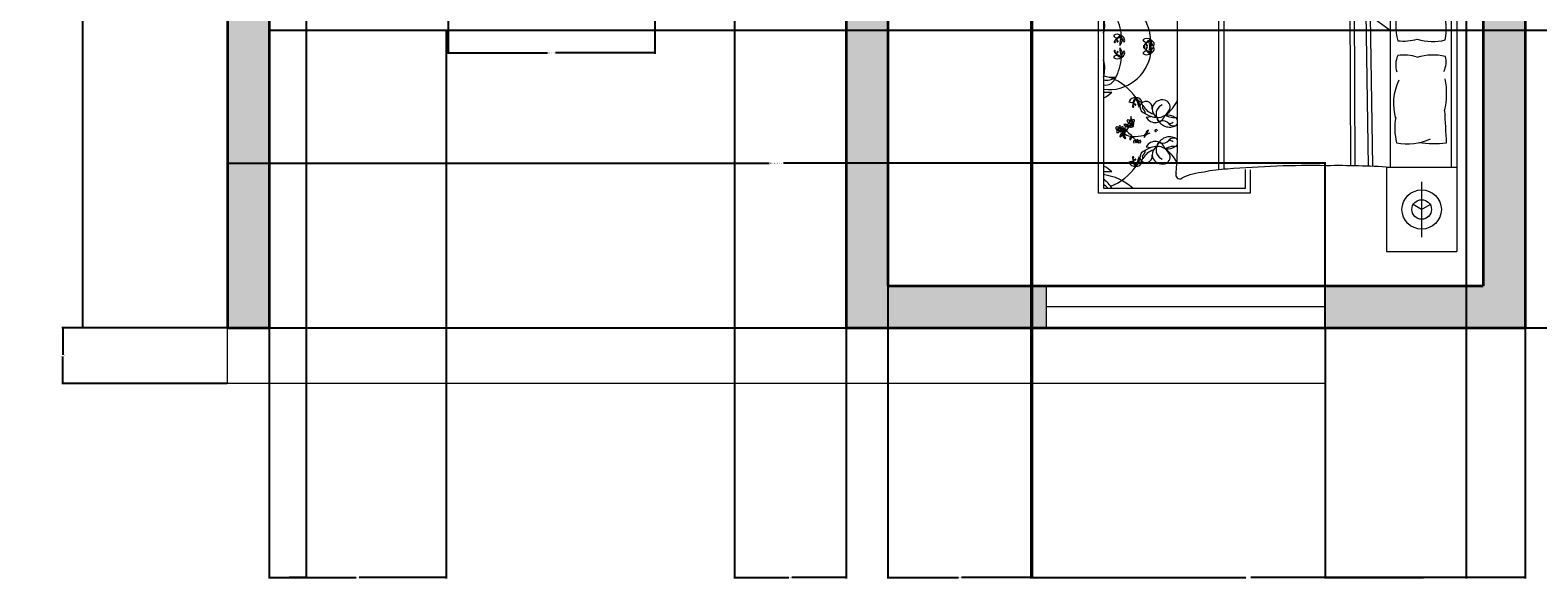
# Model space of a CAD drawing. Units: inches. Extents: x 37 to 706, y -568 to 110.
# Tile 1 of 24: x 37 to 361, y -568 to -450. Entities that reach past the tile are written whole.
import ezdxf

# ---------------------------------------------------------------- set-up
doc = ezdxf.new("R2010")
doc.units = ezdxf.units.IN
doc.header["$MEASUREMENT"] = 0
for name, color, linetype, lineweight in [('A-ANNO-DIMS', 2, 'Continuous', 18), ('A-FLOR-STRS', 7, 'Continuous', 18), ('A-FURN', 8, 'Continuous', 13), ('A-GLAZ', 4, 'Continuous', 18), ('A-WALL', 7, 'Continuous', 35), ('A-WALL-PATT', 252, 'Continuous', 13)]:
    doc.layers.add(name, color=color, linetype=linetype, lineweight=lineweight)
doc.styles.get("Standard").update_dxf_attribs({"font": 'arial.ttf'})
doc.dimstyles.get("Standard").update_dxf_attribs({"dimtxt": 0.18, "dimasz": 0.18, "dimexe": 0.18, "dimexo": 0.0625, "dimgap": 0.09, "dimtad": 0, "dimtih": 1, "dimtoh": 1, "dimdec": 0, "dimzin": 0, "dimdsep": 46, "dimlunit": 3, "dimtxsty": 'Standard', "dimcen": 0.09, "dimadec": 0, "dimazin": 0, "dimtfac": 1, "dimtdec": 0, "dimtofl": 0, "dimtmove": 0, "dimatfit": 3, "dimfxl": 1, "dimtolj": 1, "dimtzin": 0, "dimarcsym": 0})

# ---------------------------------------------------------------- blocks, each defined once
blk = doc.blocks.new('*D3')
at = {"layer": 'A-ANNO-DIMS', "color": 0, "lineweight": -2, "transparency": 16777216}
for p, q in [((78.9, 51.29), (47.67, 51.29)), ((47.85, 51.11), (47.85, -228.11)), ((47.85, -513.53), (47.85, -234.31)), ((78.9, -513.71), (47.67, -513.71))]:
    blk.add_line(p, q, dxfattribs=at)
at = {"layer": 'A-ANNO-DIMS', "color": 0, "transparency": 16777216}
for points in [[(47.82, 51.11), (47.88, 51.11), (47.85, 51.29)], [(47.82, -513.53), (47.88, -513.53), (47.85, -513.71)]]:
    blk.add_solid(points, dxfattribs=at)
at = {"layer": 'Defpoints', "color": 0, "transparency": 16777216}
for p in [(78.96, 51.29), (47.85, -513.71), (78.96, -513.71)]:
    blk.add_point(p, dxfattribs=at)
at = {"layer": 'A-ANNO-DIMS', "color": 0, "transparency": 16777216, "insert": (47.85, -231.21), "char_height": 6, "attachment_point": 5}
blk.add_mtext('\\A1;47\'-1"', dxfattribs=at)
blk = doc.blocks.new('BED-DOUBLE-WITH-NIGHTSTANDS')
for p, q in [((77.02, 90.57), (77.02, 0)), ((69.47, 75.59), (69.47, 87.43)), ((63.56, 81.51), (75.39, 81.51)), ((0, 78.61), (32.62, 78.61)), ((0, 12.59), (0, 78.61)), ((32.62, 78.61), (32.62, 73.49)), ((1.05, 77.56), (1.05, 13.64)), ((31.58, 77.56), (1.05, 77.56)), ((31.58, 73.49), (31.58, 77.56)), ((25.85, 17.62), (25.85, 73.5)), ((26.98, 17.7), (26.98, 73.5)), ((50.48, 72.53), (51.22, 73.26)), ((50.85, 68.86), (50.48, 72.53)), ((51.22, 73.26), (55.07, 69.96)), ((77.02, 72.45), (52.16, 72.45)), ((62.71, 72.45), (62.71, 18.11)), ((75.86, 18.11), (75.86, 72.45)), ((10.23, 68.64), (11.25, 68.84)), ((50.48, 64.28), (50.85, 68.86)), ((55.07, 69.96), (57.63, 66.48)), ((57.63, 66.48), (60.02, 59.87)), ((10.23, 62.31), (11.25, 62.11)), ((16.95, 26.9), (16.95, 63.67)), ((49.93, 60.24), (50.48, 64.28)), ((48.83, 57.86), (49.93, 60.24)), ((60.02, 59.87), (62.71, 50)), ((48.1, 54.92), (48.83, 57.86)), ((50.48, 54.55), (48.1, 54.92)), ((55.8, 52.54), (50.48, 54.55)), ((54.24, 18.43), (54.09, 53.18)), ((55.17, 18.44), (55.03, 52.83)), ((62.71, 47.57), (55.8, 52.54)), ((58.02, 18.39), (57.55, 51.28)), ((58.95, 18.36), (58.49, 50.6)), ((10.23, 28.89), (11.25, 29.09)), ((10.23, 22.56), (11.25, 22.36)), ((31.58, 13.64), (31.58, 17.63)), ((32.62, 17.61), (32.62, 12.59)), ((1.05, 13.64), (31.58, 13.64)), ((69.47, 14.97), (69.47, 3.14)), ((32.62, 12.59), (0, 12.59))]:
    blk.add_line(p, q)
for points in [[(61.93, 72.45), (61.93, 90.57), (77.02, 90.57)], [(69.47, 81.51), (67.64, 80.45)], [(69.47, 81.51), (71.3, 80.45)], [(77.02, 18.11), (61.93, 18.11), (61.93, 0), (77.02, 0)], [(69.47, 9.06), (67.64, 10.11)], [(69.47, 9.06), (71.3, 10.11)]]:
    blk.add_lwpolyline(points)
for points in [[(42.92, 73.45, 0.001242), (25.74, 73.5, -0.127202), (17.18, 75.31)], [(74.76, 67.25, 0.074897), (68.85, 67.14, -0.472817)], [(68.52, 45.71, 0.14099), (74.55, 45.53, 0.235245)], [(68.52, 41.84, -0.14099), (74.55, 42.02, -0.235245)], [(74.76, 23.32, -0.074897), (68.85, 23.42, 0.472817)], [(27.69, 17.73, 0.056112), (22.71, 17.07, 0.095341), (17.91, 15.8)]]:
    blk.add_lwpolyline(points, format="xyb")
for centre, radius in [((69.47, 81.51), 4.23), ((69.47, 81.51), 2.11), ((4.52, 64.91), 0.231), ((6.95, 63.41), 0.231), ((4.52, 26.28), 0.231), ((6.95, 27.79), 0.231), ((69.47, 9.06), 4.23), ((69.47, 9.06), 2.11)]:
    blk.add_circle(centre, radius)
for centre, radius, start, end in [((-3.2, 82.51), 7.18, 306.3036, 316.4814), ((-2.13, 80.43), 5.76, 303.4617, 330.1116), ((-0.54, 86.37), 11.83, 277.745, 311.8856), ((-1.71, 66.13), 11.83, 34.3865, 68.5908), ((17.23, 74.48), 0.836, 93.98, 207.3412), ((-0.79, 77.21), 4.81, 292.5547, 318.9546), ((1.79, 90.38), 16.36, 267.4081, 273.6519), ((7.77, 71.53), 1.31, 77.7115, 159.0387), ((7.06, 72.84), 0.988, 238.4633, 358.2869), ((10.3, 70.85), 2.99, 138.8402, 177.9352), ((8.5, 71.96), 0.967, 117.6827, 223.7762), ((7.89, 71.38), 0.128, 223.7762, 159.7183), ((8.28, 71.86), 0.98, 2.9516, 103.728), ((16.12, 74.61), 8.27, 192.5173, 207.1824), ((6.95, 71.3), 1.87, 345.4653, 54.2343), ((9.77, 73.87), 2.02, 211.3827, 255.2969), ((10.16, 70.71), 1.36, 350.264, 160.8688), ((8.69, 70.99), 0.833, 333.9755, 53.2681), ((13.65, 70.21), 2.16, 84.9449, 172.8857), ((14.47, 69.36), 2.1, 111.5819, 201.4221), ((13.86, 70.84), 1.53, 354.4856, 91.0538), ((10.57, 74.83), 6.85, 303.6671, 333.2997), ((-77.32, 64.75), 94.28, 359.3433, 5.6887), ((48.97, 156.3), 83.07, 265.8294, 271.553), ((83.29, 71.71), 34.18, 177.4519, 191.3392), ((7.46, 70.95), 0.147, 177.9352, 11.4834), ((7.53, 70.96), 0.0713, 11.4834, 127.9409), ((10.57, 71.04), 1.7, 175.969, 254.3045), ((8.31, 69.21), 1.81, 6.1662, 51.5825), ((13.15, 73.4), 4.28, 211.2614, 251.7045), ((12.81, 73.44), 4.86, 236.2883, 266.5076), ((12.18, 69.76), 2.25, 209.9085, 343.1337), ((14.13, 70.59), 2.63, 182.3591, 234.0401), ((12.73, 71.31), 2.72, 265.2933, 346.921), ((13.13, 68.34), 0.562, 167.3041, 285.1471), ((14.65, 65.65), 3.49, 122.7011, 126.3445), ((15.31, 69.41), 2.89, 199.2822, 299.1751), ((16.28, 72.32), 3.75, 238.8218, 279.1554), ((14.65, 65.65), 3.49, 55.785, 94.7304), ((15.95, 67.67), 1.09, 30.0293, 52.325), ((4.09, 64.6), 0.381, 61.2196, 169.0403), ((4.34, 65.38), 0.455, 157.4086, 261.4386), ((4.09, 65.4), 0.229, 58.0499, 135.6268), ((4.32, 65.26), 0.153, 172.906, 277.132), ((3.82, 64.98), 0.727, 14.7558, 58.0499), ((4.84, 65.17), 0.315, 36.1046, 181.4281), ((4.85, 66.4), 0.258, 124.3538, 214.3923), ((5.23, 66.36), 0.6, 190.3057, 287.1958), ((4.66, 65.42), 0.317, 270.0645, 331.1507), ((4.93, 65.34), 0.363, 221.8413, 265.7877), ((5.41, 66.58), 0.697, 176.9701, 248.2913), ((10.38, 70.25), 6.74, 212.6784, 216.3746), ((4.74, 64.65), 0.22, 1.1081, 91.8675), ((4.92, 65.2), 0.226, 263.7526, 41.7054), ((4.88, 64.6), 0.385, 11.5637, 86.365), ((5.17, 66.41), 0.267, 216.3746, 291.7548), ((7.53, 62.67), 3.76, 124.0033, 132.4917), ((3.66, 62.2), 4.02, 63.7819, 68.2913), ((5.81, 65.29), 0.639, 128.3208, 208.8162), ((5.81, 66.23), 0.6, 122.8155, 187.3992), ((5.92, 65.34), 0.764, 207.7043, 254.3516), ((5.34, 65.98), 0.201, 289.3605, 111.7548), ((5.49, 65.98), 0.201, 221.8703, 44.2646), ((6.41, 65.39), 1.05, 157.2305, 229.0635), ((6.07, 66.15), 0.697, 109.4799, 177.6828), ((6.05, 65.74), 0.619, 174.4544, 220.6188), ((2.53, 62.29), 4.51, 30.544, 49.818), ((5.7, 66.59), 0.258, 56.8636, 146.9021), ((5.83, 66.31), 0.267, 148.8844, 224.2646), ((5.02, 64.86), 0.744, 340.0041, 40.6188), ((11.37, 62.96), 6.74, 145.1882, 148.8844), ((7.53, 62.67), 3.76, 94.756, 119.2041), ((15.54, 57.26), 12.37, 132.2412, 142.1744), ((9.29, 67.11), 2.55, 178.3264, 187.1302), ((6.53, 66.75), 0.476, 11.3256, 64.4621), ((8.15, 67.44), 1.43, 190.2588, 210.656), ((7.19, 66.85), 0.435, 188.3432, 274.2869), ((7.57, 67.09), 0.759, 210.656, 242.6341), ((8.14, 67.75), 1.46, 218.2101, 226.3071), ((7.07, 66.52), 0.185, 325.7657, 67.4417), ((1.34, 72.69), 8.6, 313.1541, 322.0459), ((7.72, 58.94), 7.5, 73.5842, 93.8277), ((7.66, 67.53), 0.177, 142.4737, 265.053), ((7.89, 67.56), 0.381, 127.7621, 169.0403), ((7.69, 67.89), 0.536, 265.053, 338.3618), ((8.4, 67.15), 0.7, 113.4276, 137.6104), ((8.32, 67.88), 0.231, 183.2768, 356.7232), ((8.49, 67.46), 0.377, 139.7889, 227.6792), ((8.37, 67.33), 0.199, 227.6792, 350.3487), ((7.6, 67.46), 0.755, 353.0852, 15.7171), ((8.1, 67.37), 0.477, 350.3487, 43.6538), ((8.98, 67.87), 0.555, 198.7263, 262.5032), ((8.54, 67.61), 0.22, 1.1081, 91.8675), ((8.68, 67.56), 0.385, 11.5637, 52.6358), ((8.95, 67.49), 0.178, 255.2356, 54.9248), ((12.34, 66.57), 2.55, 178.3264, 187.1302), ((9.58, 66.21), 0.476, 11.3256, 64.4621), ((11.19, 66.9), 1.43, 190.2588, 210.656), ((10.23, 66.31), 0.435, 188.3432, 274.2869), ((10.61, 66.55), 0.759, 210.656, 242.6341), ((11.19, 67.21), 1.46, 218.2101, 226.3071), ((10.11, 65.98), 0.185, 325.7657, 67.4417), ((10.63, 65.65), 0.435, 147.5332, 233.4768), ((11.02, 65.87), 0.759, 179.1859, 211.164), ((10.28, 65.7), 0.185, 354.3784, 96.0543), ((7.72, 58.94), 7.5, 63.0032, 69.8941), ((11.6, 66.22), 1.43, 211.164, 231.5612), ((11.85, 67.38), 2.55, 234.6898, 243.4936), ((11.87, 66.07), 1.46, 195.5129, 203.6099), ((10.23, 65.12), 0.476, 357.3579, 50.4944), ((12.28, 65.21), 0.175, 12.7051, 190.4384), ((12.38, 65.23), 0.284, 190.4384, 10.4136), ((13.76, 66), 1.86, 41.5653, 105.1471), ((14.78, 69.85), 2.6, 277.436, 299.9149), ((16.16, 68.13), 1.36, 221.5653, 293.8354), ((15.95, 67.67), 1.09, 314.4517, 333.558), ((42.55, 63.54), 7.37, 336.2616, 11.3392), ((75.82, 64.02), 12.14, 165.1039, 191.0369), ((66.47, 55.71), 11.67, 65.1316, 101.7583), ((936.66, 17.33), 863.34, 176.68521, 177.14978), ((3.86, 64.56), 0.177, 142.4737, 265.053), ((3.89, 64.92), 0.536, 265.053, 338.3618), ((4.6, 64.19), 0.7, 113.4276, 137.6104), ((4.69, 64.5), 0.377, 139.7889, 227.6792), ((4.57, 64.37), 0.199, 227.6792, 350.3487), ((3.8, 64.5), 0.755, 353.0852, 15.7171), ((4.29, 64.41), 0.477, 350.3487, 43.6538), ((5.18, 64.9), 0.555, 198.7263, 262.5032), ((5.15, 64.53), 0.178, 255.2356, 54.9248), ((5.43, 64.9), 1.05, 270.278, 342.111), ((6.13, 63.58), 0.744, 98.7227, 159.3375), ((5.75, 64.54), 0.764, 244.9899, 291.6373), ((5.92, 64.93), 0.619, 278.7227, 324.8872), ((5.81, 64.43), 0.639, 290.5253, 358.5375), ((6.29, 63.06), 0.177, 142.4737, 265.053), ((6.52, 63.09), 0.381, 61.2196, 169.0403), ((6.32, 63.41), 0.536, 265.053, 338.3618), ((6.77, 63.88), 0.455, 157.4086, 261.4386), ((6.52, 63.89), 0.229, 58.0499, 135.6268), ((7.06, 64.61), 0.639, 182.8499, 266.1226), ((6.81, 65.06), 0.619, 231.7607, 277.9252), ((7.29, 65.17), 1.05, 214.5369, 286.3699), ((7.03, 62.68), 0.7, 113.4276, 137.6104), ((6.76, 63.75), 0.153, 172.906, 277.132), ((6.25, 63.47), 0.727, 14.7558, 58.0499), ((2.53, 62.29), 4.51, 23.0501, 23.8477), ((7.12, 62.99), 0.377, 139.7889, 227.6792), ((7, 62.86), 0.199, 227.6792, 350.3487), ((7, 63.71), 0.744, 37.3105, 97.9252), ((7.27, 63.66), 0.315, 36.1046, 181.4281), ((6.23, 62.99), 0.755, 353.0852, 15.7171), ((7.08, 64.73), 0.764, 265.0106, 311.658), ((2.53, 62.29), 4.51, 357.1071, 4.7585), ((6.72, 62.9), 0.477, 350.3487, 43.6538), ((7.61, 63.4), 0.555, 198.7263, 262.5032), ((7.09, 63.91), 0.317, 270.0645, 331.1507), ((7.36, 63.83), 0.363, 221.8413, 265.7877), ((7.17, 63.14), 0.22, 1.1081, 91.8675), ((7.36, 63.7), 0.226, 263.7526, 41.7054), ((7.31, 63.09), 0.385, 11.5637, 86.365), ((7.58, 63.02), 0.178, 255.2356, 54.9248), ((13.15, 57.54), 4.28, 108.2955, 148.7386), ((12.81, 57.5), 4.86, 93.4924, 123.7117), ((12.18, 61.19), 2.25, 16.8663, 150.0915), ((14.13, 60.36), 2.63, 125.9599, 177.6409), ((14.47, 61.59), 2.1, 158.5779, 248.4181), ((12.73, 59.64), 2.72, 13.079, 94.7067), ((13.13, 62.61), 0.562, 74.8529, 192.6959), ((15.31, 61.54), 2.89, 60.8249, 160.7178), ((14.65, 65.3), 3.49, 233.6555, 237.2989), ((13.76, 64.95), 1.86, 254.8529, 318.4347), ((16.28, 58.63), 3.75, 79.7133, 121.1782), ((14.65, 65.3), 3.49, 265.2696, 304.215), ((10.57, 56.11), 6.85, 21.4941, 56.3329), ((14.78, 61.1), 2.6, 60.0851, 82.564), ((16.16, 62.82), 1.36, 66.1646, 138.4347), ((15.95, 63.28), 1.09, 307.675, 336.7144), ((15.95, 63.28), 1.09, 23.229, 45.5483), ((84.45, 57.63), 21.05, 168.0397, 199.2615), ((7.06, 58.1), 0.988, 1.7131, 121.5367), ((7.77, 59.41), 1.31, 200.9613, 282.2885), ((7.46, 60), 0.147, 348.5166, 182.0648), ((10.3, 60.1), 2.99, 182.0648, 221.1598), ((7.53, 59.98), 0.0713, 232.0591, 348.5166), ((8.5, 58.99), 0.967, 136.2238, 242.3173), ((7.94, 59.56), 0.0771, 200.2667, 136.2271), ((6.95, 59.65), 1.87, 305.7657, 14.5347), ((16.12, 56.34), 8.27, 152.8176, 167.4827), ((8.28, 59.09), 0.98, 256.272, 357.0484), ((9.77, 57.08), 2.02, 104.7031, 148.6173), ((10.57, 59.91), 1.7, 105.6955, 184.031), ((10.16, 60.24), 1.36, 199.1312, 9.736), ((8.69, 59.96), 0.833, 306.7319, 26.0245), ((8.31, 61.74), 1.81, 308.4175, 353.8338), ((13.65, 60.74), 2.16, 187.1143, 275.0551), ((13.86, 60.11), 1.53, 268.9462, 5.5144), ((82.33, 48.63), 35.12, 160.1194, 169.3383), ((41.99, 54.84), 32.85, 352.2196, 9.497), ((-0.79, 53.74), 4.81, 41.0454, 67.4453), ((1.79, 40.57), 16.36, 86.3481, 92.5919), ((-0.54, 44.58), 11.83, 4.4623, 82.255), ((-2.13, 50.51), 5.76, 1.272, 56.5383), ((-1.71, 64.81), 11.83, 291.4092, 325.6135), ((48.03, 55.13), 0.219, 178.8623, 289.7536), ((-3.2, 48.44), 7.18, 17.8504, 53.6964), ((-5.22, 44.66), 10.68, 34.0123, 54.053), ((79.85, 49.11), 15.97, 169.8617, 193.6238), ((-5.17, 48.79), 6.5, 343.5431, 17.0202), ((-6.88, 45.48), 11.83, 4.4623, 27.4146), ((58.59, 47.9), 16.14, 351.5249, 13.96), ((-8.52, 46.22), 9.62, 4.3787, 5.6357), ((-15.11, 41.15), 17.18, 19.7217, 19.9028), ((4.03, 45.43), 1.31, 47.7873, 129.1145), ((4.07, 46.92), 0.988, 208.5391, 328.3627), ((5.88, 43.58), 2.99, 108.9159, 148.011), ((4.87, 45.44), 0.967, 87.7585, 193.852), ((12.81, 43.93), 8.27, 162.593, 177.2582), ((3.21, 45.64), 1.87, 315.5411, 24.3101), ((6.93, 46.46), 2.02, 181.4585, 225.3727), ((4.64, 45.46), 0.98, 333.0274, 73.8037), ((10.37, 44.53), 1.31, 47.7873, 129.1145), ((10.41, 46.02), 0.988, 208.5391, 328.3627), ((12.22, 42.67), 2.99, 108.9159, 148.011), ((11.21, 44.53), 0.967, 87.7585, 193.852), ((9.54, 44.73), 1.87, 315.5411, 24.3101), ((19.14, 43.02), 8.27, 162.593, 177.2582), ((10.97, 44.56), 0.98, 333.0274, 73.8037), ((13.27, 45.55), 2.02, 181.4585, 225.3727), ((65.49, 56.38), 11.1, 264.0129, 285.8293), ((2.19, 43.98), 9.15, 262.8636, 351.8197), ((4.07, 41.26), 0.988, 31.6373, 151.4609), ((3.47, 45.08), 0.147, 148.011, 341.5592), ((3.47, 43.1), 0.147, 18.4408, 211.989), ((5.88, 44.6), 2.99, 211.989, 251.0841), ((3.54, 45.06), 0.0713, 341.5592, 98.0167), ((3.54, 43.12), 0.0713, 261.9833, 18.4408), ((4.87, 42.74), 0.967, 166.148, 272.2415), ((4.06, 45.24), 0.128, 193.852, 129.9245), ((4.11, 42.95), 0.0771, 230.1909, 166.0209), ((12.81, 44.25), 8.27, 182.7418, 197.407), ((3.21, 42.54), 1.87, 335.6899, 44.4589), ((6.93, 41.72), 2.02, 134.6273, 178.5415), ((4.64, 42.72), 0.98, 286.1963, 26.9726), ((10.41, 42.16), 0.988, 31.6373, 151.4609), ((10.37, 43.65), 1.31, 230.8855, 312.2127), ((9.8, 44.18), 0.147, 148.011, 341.5592), ((9.8, 44), 0.147, 18.4408, 211.989), ((12.22, 45.51), 2.99, 211.989, 251.0841), ((9.88, 44.15), 0.0713, 341.5592, 98.0167), ((9.88, 44.03), 0.0713, 261.9833, 18.4408), ((11.21, 43.65), 0.967, 166.148, 272.2415), ((10.39, 44.33), 0.128, 193.852, 129.9245), ((10.44, 43.86), 0.0771, 230.1909, 166.0209), ((9.54, 43.45), 1.87, 335.6899, 44.4589), ((19.14, 45.16), 8.27, 182.7418, 197.407), ((10.97, 43.62), 0.98, 286.1963, 26.9726), ((13.27, 42.63), 2.02, 134.6273, 178.5415), ((68.68, 40.17), 4.8, 155.0183, 198.5407), ((65.49, 31.16), 11.1, 74.1707, 95.9871), ((-5.17, 39.39), 6.5, 342.9798, 16.4569), ((-8.52, 41.96), 9.62, 354.3643, 355.6213), ((-15.11, 47.03), 17.18, 340.0972, 340.2783), ((4.03, 42.75), 1.31, 230.8855, 312.2127), ((-6.88, 42.69), 11.83, 332.5854, 355.5377), ((70.25, 40.78), 4.48, 333.3437, 16.1026), ((3.02, 42.8), 5.3, 248.117, 276.6195), ((1.55, 37.94), 2.12, 256.3898, 349.0739), ((1.84, 39.54), 2.68, 252.8609, 311.9049), ((-1.71, 26.39), 11.83, 34.3865, 68.5908), ((74.93, 31.78), 11.53, 153.8761, 196.1746), ((58.92, 34.06), 15.92, 346.3427, 11.1841), ((1.79, 50.63), 16.36, 267.4081, 273.6519), ((-0.79, 37.46), 4.81, 292.5547, 318.9546), ((7.77, 31.78), 1.31, 77.7115, 159.0387), ((7.06, 33.09), 0.988, 238.4633, 358.2869), ((10.3, 31.1), 2.99, 138.8402, 177.9352), ((8.5, 32.21), 0.967, 117.6827, 223.7762), ((8.28, 32.11), 0.98, 2.9516, 103.728), ((9.77, 34.12), 2.02, 211.3827, 255.2969), ((6.95, 31.55), 1.87, 345.4653, 54.2343), ((16.12, 34.86), 8.27, 192.5173, 207.1824), ((13.65, 30.46), 2.16, 84.9449, 172.8857), ((13.86, 31.09), 1.53, 354.4856, 91.0538), ((10.57, 35.08), 6.85, 303.6671, 338.5059), ((7.46, 31.2), 0.147, 177.9352, 11.4834), ((7.53, 31.21), 0.0713, 11.4834, 127.9409), ((7.89, 31.63), 0.128, 223.7762, 159.7183), ((10.16, 30.96), 1.36, 350.264, 160.8688), ((10.57, 31.29), 1.7, 175.969, 254.3045), ((8.69, 31.24), 0.833, 333.9755, 53.2681), ((8.31, 29.46), 1.81, 6.1662, 51.5825), ((13.15, 33.66), 4.28, 211.2614, 251.7045), ((12.81, 33.7), 4.86, 236.2883, 266.5076), ((12.18, 30.01), 2.25, 209.9085, 343.1337), ((14.13, 30.84), 2.63, 182.3591, 234.0401), ((14.47, 29.61), 2.1, 111.5819, 201.4221), ((12.73, 31.56), 2.72, 265.2933, 346.921), ((16.28, 32.57), 3.75, 238.8218, 280.2867), ((14.65, 25.9), 3.49, 55.785, 94.7304), ((936.66, 73.23), 863.34, 182.85022, 183.31479), ((3.86, 26.63), 0.177, 94.947, 217.5263), ((4.09, 26.6), 0.381, 190.9597, 298.7804), ((3.89, 26.28), 0.536, 21.6382, 94.947), ((4.34, 25.81), 0.455, 98.5614, 202.5914), ((4.6, 27.01), 0.7, 222.3896, 246.5724), ((4.32, 25.94), 0.153, 82.868, 187.094), ((3.82, 26.22), 0.727, 301.9501, 345.2442), ((4.69, 26.7), 0.377, 132.3208, 220.2111), ((4.57, 26.83), 0.199, 9.6513, 132.3208), ((4.84, 26.03), 0.315, 178.5719, 323.8954), ((3.8, 26.7), 0.755, 344.2829, 6.9148), ((4.29, 26.79), 0.477, 316.3462, 9.6513), ((5.18, 26.29), 0.555, 97.4968, 161.2737), ((4.93, 25.86), 0.363, 94.2123, 138.1587), ((4.66, 25.78), 0.317, 28.8493, 89.9355), ((4.74, 26.55), 0.22, 268.1325, 358.8919), ((4.88, 26.6), 0.385, 273.635, 348.4363), ((4.92, 25.99), 0.226, 318.2946, 96.2474), ((5.15, 26.67), 0.178, 305.0752, 104.7644), ((5.81, 25.91), 0.639, 151.1838, 231.6792), ((5.92, 25.86), 0.764, 105.6484, 152.2957), ((6.41, 25.8), 1.05, 130.9365, 202.7695), ((5.75, 26.66), 0.764, 68.3627, 115.0101), ((5.43, 26.3), 1.05, 17.889, 89.722), ((6.13, 27.61), 0.744, 200.6625, 261.2773), ((2.53, 28.91), 4.51, 310.182, 329.456), ((5.02, 26.34), 0.744, 319.3812, 19.9959), ((15.54, 33.94), 12.37, 217.8256, 227.7588), ((5.92, 26.27), 0.619, 35.1128, 81.2773), ((5.81, 26.77), 0.639, 1.4625, 69.4747), ((6.29, 28.14), 0.177, 94.947, 217.5263), ((6.52, 28.11), 0.381, 190.9597, 298.7804), ((6.32, 27.78), 0.536, 21.6382, 94.947), ((6.77, 27.32), 0.455, 98.5614, 202.5914), ((6.52, 27.31), 0.229, 224.3732, 301.9501), ((7.06, 26.59), 0.639, 93.8774, 177.1501), ((7.29, 26.03), 1.05, 73.6301, 145.4631), ((6.81, 26.14), 0.619, 82.0748, 128.2393), ((7.03, 28.52), 0.7, 222.3896, 246.5724), ((6.76, 27.45), 0.153, 82.868, 187.094), ((6.25, 27.73), 0.727, 301.9501, 345.2442), ((2.53, 28.91), 4.51, 336.1523, 336.9499), ((7.12, 28.21), 0.377, 132.3208, 220.2111), ((7, 28.34), 0.199, 9.6513, 132.3208), ((7, 27.49), 0.744, 262.0748, 322.6895), ((6.23, 28.2), 0.755, 344.2829, 6.9148), ((7.27, 27.54), 0.315, 178.5719, 323.8954), ((7.08, 26.46), 0.764, 48.342, 94.9894), ((2.53, 28.91), 4.51, 355.2415, 2.8929), ((6.72, 28.3), 0.477, 316.3462, 9.6513), ((7.61, 27.8), 0.555, 97.4968, 161.2737), ((7.36, 27.37), 0.363, 94.2123, 138.1587), ((7.09, 27.29), 0.317, 28.8493, 89.9355), ((7.17, 28.06), 0.22, 268.1325, 358.8919), ((7.31, 28.11), 0.385, 273.635, 348.4363), ((7.36, 27.5), 0.226, 318.2946, 96.2474), ((7.58, 28.18), 0.178, 305.0752, 104.7644), ((11.6, 24.98), 1.43, 128.4388, 148.836), ((11.85, 23.82), 2.55, 116.5064, 125.3102), ((10.23, 26.08), 0.476, 309.5056, 2.6421), ((12.28, 25.98), 0.175, 169.5616, 347.2949), ((12.38, 25.96), 0.284, 349.5864, 169.5616), ((13.13, 28.59), 0.562, 167.3041, 285.1471), ((14.65, 25.9), 3.49, 122.7011, 126.3445), ((15.31, 29.66), 2.89, 199.2822, 299.1751), ((13.76, 26.25), 1.86, 41.5653, 105.1471), ((14.78, 30.1), 2.6, 277.436, 299.9149), ((16.16, 28.38), 1.36, 221.5653, 293.8354), ((15.95, 27.92), 1.09, 23.2856, 52.325), ((-71.13, 24.12), 88.13, 355.2402, 1.8035), ((15.95, 27.92), 1.09, 314.4517, 336.7144), ((75.82, 26.55), 12.14, 168.9631, 194.8961), ((4.09, 25.8), 0.229, 224.3732, 301.9501), ((4.85, 24.8), 0.258, 145.6077, 235.6462), ((5.23, 24.83), 0.6, 72.8042, 169.6943), ((5.41, 24.62), 0.697, 111.7087, 183.0299), ((10.38, 20.95), 6.74, 143.6254, 147.3216), ((5.17, 24.78), 0.267, 68.2452, 143.6254), ((7.53, 28.53), 3.76, 227.5083, 235.9967), ((3.66, 29), 4.02, 291.7087, 296.2181), ((5.81, 24.97), 0.6, 172.6008, 237.1845), ((5.34, 25.22), 0.201, 248.2452, 70.6395), ((5.49, 25.22), 0.201, 315.7354, 138.1297), ((6.07, 25.05), 0.697, 182.3172, 250.5201), ((6.05, 25.46), 0.619, 139.3812, 185.5456), ((5.7, 24.61), 0.258, 213.0979, 303.1364), ((5.83, 24.89), 0.267, 135.7354, 211.1156), ((11.37, 28.24), 6.74, 211.1156, 214.8118), ((7.53, 28.53), 3.76, 240.7959, 265.244), ((8.15, 23.76), 1.43, 149.344, 169.7412), ((9.29, 24.09), 2.55, 172.8698, 181.6736), ((6.53, 24.45), 0.476, 295.5379, 348.6744), ((7.19, 24.34), 0.435, 85.7131, 171.6568), ((7.57, 24.1), 0.759, 117.3659, 149.344), ((8.14, 23.45), 1.46, 133.6929, 141.7899), ((7.07, 24.67), 0.185, 292.5583, 34.2343), ((7.72, 32.26), 7.5, 266.1723, 286.4158), ((1.34, 18.5), 8.6, 37.9541, 46.8459), ((7.66, 23.67), 0.177, 94.947, 217.5263), ((7.89, 23.64), 0.381, 190.9597, 232.2379), ((7.69, 23.31), 0.536, 21.6382, 94.947), ((8.4, 24.05), 0.7, 222.3896, 246.5724), ((8.32, 23.32), 0.231, 3.2768, 176.7232), ((8.49, 23.74), 0.377, 132.3208, 220.2111), ((8.37, 23.87), 0.199, 9.6513, 132.3208), ((7.6, 23.73), 0.755, 344.2829, 6.9148), ((8.1, 23.82), 0.477, 316.3462, 9.6513), ((8.98, 23.33), 0.555, 97.4968, 161.2737), ((8.54, 23.59), 0.22, 268.1325, 358.8919), ((8.95, 23.71), 0.178, 305.0752, 104.7644), ((8.68, 23.64), 0.385, 307.3642, 348.4363), ((11.19, 24.3), 1.43, 149.344, 169.7412), ((12.34, 24.63), 2.55, 172.8698, 181.6736), ((9.58, 24.98), 0.476, 295.5379, 348.6744), ((10.23, 24.88), 0.435, 85.7131, 171.6568), ((10.61, 24.64), 0.759, 117.3659, 149.344), ((11.19, 23.99), 1.46, 133.6929, 141.7899), ((10.11, 25.21), 0.185, 292.5583, 34.2343), ((10.63, 25.55), 0.435, 126.5232, 212.4668), ((12.18, 21.44), 2.25, 16.8663, 150.0915), ((11.02, 25.33), 0.759, 148.836, 180.8141), ((10.28, 25.5), 0.185, 263.9457, 5.6216), ((7.72, 32.26), 7.5, 290.1059, 296.9968), ((11.87, 25.13), 1.46, 156.3901, 164.4871), ((14.13, 20.61), 2.63, 125.9599, 177.6409), ((13.13, 22.86), 0.562, 74.8529, 192.6959), ((15.31, 21.79), 2.89, 60.8249, 160.7178), ((14.65, 25.55), 3.49, 233.6555, 237.2989), ((13.76, 25.2), 1.86, 254.8529, 318.4347), ((14.78, 21.35), 2.6, 60.0851, 82.564), ((16.16, 23.07), 1.36, 66.1646, 138.4347), ((15.95, 23.53), 1.09, 307.675, 342.5814), ((15.95, 23.53), 1.09, 16.6343, 45.5483), ((66.47, 34.85), 11.67, 258.2417, 294.8684), ((7.46, 20.25), 0.147, 348.5166, 182.0648), ((10.3, 20.35), 2.99, 182.0648, 221.1598), ((7.53, 20.24), 0.0713, 232.0591, 348.5166), ((8.5, 19.24), 0.967, 136.2238, 242.3173), ((7.94, 19.81), 0.0771, 200.2667, 136.2271), ((16.12, 16.59), 8.27, 152.8176, 167.4827), ((6.95, 19.9), 1.87, 305.7657, 14.5347), ((10.57, 20.16), 1.7, 105.6955, 184.031), ((10.16, 20.49), 1.36, 199.1312, 9.736), ((8.69, 20.21), 0.833, 306.7319, 26.0245), ((8.31, 21.99), 1.81, 308.4175, 353.8338), ((13.15, 17.79), 4.28, 108.2955, 148.7386), ((12.81, 17.75), 4.86, 93.4924, 123.7117), ((13.65, 20.99), 2.16, 187.1143, 275.0551), ((14.47, 21.84), 2.1, 158.5779, 248.4181), ((12.73, 19.89), 2.72, 13.079, 94.7067), ((13.86, 20.36), 1.53, 268.9462, 5.5144), ((16.28, 18.88), 3.75, 79.249, 121.1782), ((14.65, 25.55), 3.49, 265.2696, 304.215), ((10.57, 16.37), 6.85, 23.6453, 56.3329), ((-0.79, 13.99), 4.81, 41.0454, 67.4453), ((1.79, 0.82), 16.36, 86.3481, 92.5919), ((-0.54, 4.83), 11.83, 48.1144, 82.255), ((-1.71, 25.06), 11.83, 291.4092, 325.6135), ((7.06, 18.36), 0.988, 1.7131, 121.5367), ((7.77, 19.67), 1.31, 200.9613, 282.2885), ((9.77, 17.33), 2.02, 104.7031, 148.6173), ((8.28, 19.34), 0.98, 256.272, 357.0484), ((17.45, 16.48), 0.826, 156.5219, 303.8264), ((45.72, -193.78), 212.28, 89.1145, 94.8735), ((51.64, -144.24), 162.73, 86.1, 90.9282), ((-2.13, 10.76), 5.76, 29.8884, 56.5383), ((-3.2, 8.69), 7.18, 43.5186, 53.6964)]:
    blk.add_arc(centre, radius, start, end)
blk = doc.blocks.new('WIN-60')
for p, q in [((60, 9), (0, 9)), ((0, 9), (0, 0)), ((60, 0), (60, 9)), ((60, 4.5), (0, 4.5)), ((0, 0), (60, 0))]:
    blk.add_line(p, q)
blk = doc.blocks.new('ENTRY-STEP-236')
for p, q in [((0, 0), (0, 12)), ((236, 12), (236, 0)), ((236, 0), (0, 0))]:
    blk.add_line(p, q)
blk = doc.blocks.new('*D30')
at = {"layer": 'A-ANNO-DIMS', "color": 0, "lineweight": -2, "transparency": 16777216}
for p, q in [((126.43, -440.85), (126.43, -454.79)), ((170.85, -440.85), (170.85, -454.79)), ((126.61, -454.61), (147.79, -454.61)), ((170.67, -454.61), (149.49, -454.61))]:
    blk.add_line(p, q, dxfattribs=at)
at = {"layer": 'A-ANNO-DIMS', "color": 0, "transparency": 16777216}
for points in [[(126.61, -454.58), (126.61, -454.64), (126.43, -454.61)], [(170.67, -454.58), (170.67, -454.64), (170.85, -454.61)]]:
    blk.add_solid(points, dxfattribs=at)
at = {"layer": 'Defpoints', "color": 0, "transparency": 16777216}
for p in [(126.43, -440.79), (170.85, -440.79), (170.85, -454.61)]:
    blk.add_point(p, dxfattribs=at)
at = {"layer": 'A-ANNO-DIMS', "color": 0, "transparency": 16777216, "insert": (148.64, -454.61), "char_height": 0.18, "attachment_point": 5}
blk.add_mtext('\\A1;3\'-8 1/2" TYP.', dxfattribs=at)
blk = doc.blocks.new('*D39')
at = {"layer": 'A-ANNO-DIMS', "color": 0, "lineweight": -2, "transparency": 16777216}
for p, q in [((78.96, -513.65), (78.96, -478.13)), ((79.14, -478.31), (195.43, -478.31)), ((314.78, -478.31), (198.49, -478.31)), ((314.96, -513.65), (314.96, -478.13))]:
    blk.add_line(p, q, dxfattribs=at)
at = {"layer": 'A-ANNO-DIMS', "color": 0, "transparency": 16777216}
for points in [[(79.14, -478.28), (79.14, -478.34), (78.96, -478.31)], [(314.78, -478.28), (314.78, -478.34), (314.96, -478.31)]]:
    blk.add_solid(points, dxfattribs=at)
at = {"layer": 'Defpoints', "color": 0, "transparency": 16777216}
for p in [(314.96, -478.31), (78.96, -513.71), (314.96, -513.71)]:
    blk.add_point(p, dxfattribs=at)
at = {"layer": 'A-ANNO-DIMS', "color": 0, "transparency": 16777216, "insert": (196.96, -478.31), "char_height": 0.18, "attachment_point": 5}
blk.add_mtext('\\A1;ENTRY STEP 19\'-8" TYP.', dxfattribs=at)
blk = doc.blocks.new('*D40')
at = {"layer": 'A-ANNO-DIMS', "color": 0, "lineweight": -2, "transparency": 16777216}
for p, q in [((78.9, -513.71), (43.38, -513.71)), ((43.56, -513.89), (43.56, -519.53)), ((43.56, -525.53), (43.56, -519.89)), ((78.9, -525.71), (43.38, -525.71))]:
    blk.add_line(p, q, dxfattribs=at)
at = {"layer": 'A-ANNO-DIMS', "color": 0, "transparency": 16777216}
for points in [[(43.53, -513.89), (43.59, -513.89), (43.56, -513.71)], [(43.53, -525.53), (43.59, -525.53), (43.56, -525.71)]]:
    blk.add_solid(points, dxfattribs=at)
at = {"layer": 'Defpoints', "color": 0, "transparency": 16777216}
for p in [(43.56, -513.71), (78.96, -513.71), (78.96, -525.71)]:
    blk.add_point(p, dxfattribs=at)
at = {"layer": 'A-ANNO-DIMS', "color": 0, "transparency": 16777216, "insert": (43.56, -519.71), "char_height": 0.18, "attachment_point": 5}
blk.add_mtext('\\A1;1\'-0" TYP.', dxfattribs=at)
blk = doc.blocks.new('*D43')
at = {"layer": 'A-ANNO-DIMS', "color": 0, "lineweight": -2, "transparency": 16777216}
for p, q in [((87.96, -449.77), (87.96, -567.64)), ((125.96, -449.77), (125.96, -567.64)), ((88.14, -567.46), (106.63, -567.46)), ((125.78, -567.46), (107.29, -567.46))]:
    blk.add_line(p, q, dxfattribs=at)
at = {"layer": 'A-ANNO-DIMS', "color": 0, "transparency": 16777216}
for points in [[(88.14, -567.43), (88.14, -567.49), (87.96, -567.46)], [(125.78, -567.43), (125.78, -567.49), (125.96, -567.46)]]:
    blk.add_solid(points, dxfattribs=at)
at = {"layer": 'Defpoints', "color": 0, "transparency": 16777216}
for p in [(87.96, -449.71), (125.96, -449.71), (125.96, -567.46)]:
    blk.add_point(p, dxfattribs=at)
at = {"layer": 'A-ANNO-DIMS', "color": 0, "transparency": 16777216, "insert": (106.96, -567.46), "char_height": 0.18, "attachment_point": 5}
blk.add_mtext('\\A1;3\'-2"', dxfattribs=at)
blk = doc.blocks.new('*D45')
at = {"layer": 'A-ANNO-DIMS', "color": 0, "lineweight": -2, "transparency": 16777216}
for p, q in [((88.02, -449.71), (705.89, -449.71)), ((705.71, -449.89), (705.71, -481.53)), ((705.71, -513.53), (705.71, -481.89)), ((79.02, -513.71), (705.89, -513.71))]:
    blk.add_line(p, q, dxfattribs=at)
at = {"layer": 'A-ANNO-DIMS', "color": 0, "transparency": 16777216}
for points in [[(705.68, -449.89), (705.74, -449.89), (705.71, -449.71)], [(705.68, -513.53), (705.74, -513.53), (705.71, -513.71)]]:
    blk.add_solid(points, dxfattribs=at)
at = {"layer": 'Defpoints', "color": 0, "transparency": 16777216}
for p in [(87.96, -449.71), (705.71, -449.71), (78.96, -513.71)]:
    blk.add_point(p, dxfattribs=at)
at = {"layer": 'A-ANNO-DIMS', "color": 0, "transparency": 16777216, "insert": (705.71, -481.71), "char_height": 0.18, "attachment_point": 5}
blk.add_mtext('\\A1;5\'-4"', dxfattribs=at)
blk = doc.blocks.new('*D47')
at = {"layer": 'A-ANNO-DIMS', "color": 0, "lineweight": -2, "transparency": 16777216}
for p, q in [((314.96, -513.77), (314.96, -567.64)), ((357.96, -513.77), (357.96, -567.64)), ((315.14, -567.46), (336.13, -567.46)), ((357.78, -567.46), (336.79, -567.46))]:
    blk.add_line(p, q, dxfattribs=at)
at = {"layer": 'A-ANNO-DIMS', "color": 0, "transparency": 16777216}
for points in [[(315.14, -567.43), (315.14, -567.49), (314.96, -567.46)], [(357.78, -567.43), (357.78, -567.49), (357.96, -567.46)]]:
    blk.add_solid(points, dxfattribs=at)
at = {"layer": 'Defpoints', "color": 0, "transparency": 16777216}
for p in [(314.96, -513.71), (357.96, -513.71), (314.96, -567.46)]:
    blk.add_point(p, dxfattribs=at)
at = {"layer": 'A-ANNO-DIMS', "color": 0, "transparency": 16777216, "insert": (336.46, -567.46), "char_height": 0.18, "attachment_point": 5}
blk.add_mtext('\\A1;3\'-7"', dxfattribs=at)
blk = doc.blocks.new('*D49')
at = {"layer": 'A-ANNO-DIMS', "color": 0, "lineweight": -2, "transparency": 16777216}
for p, q in [((251.66, -266.36), (251.66, -567.64)), ((345.27, -266.36), (345.27, -567.64)), ((251.84, -567.46), (297.93, -567.46)), ((345.09, -567.46), (299, -567.46))]:
    blk.add_line(p, q, dxfattribs=at)
at = {"layer": 'A-ANNO-DIMS', "color": 0, "transparency": 16777216}
for points in [[(251.84, -567.43), (251.84, -567.49), (251.66, -567.46)], [(345.09, -567.43), (345.09, -567.49), (345.27, -567.46)]]:
    blk.add_solid(points, dxfattribs=at)
at = {"layer": 'Defpoints', "color": 0, "transparency": 16777216}
for p in [(251.66, -266.29), (345.27, -266.29), (345.27, -567.46)]:
    blk.add_point(p, dxfattribs=at)
at = {"layer": 'A-ANNO-DIMS', "color": 0, "transparency": 16777216, "insert": (298.47, -567.46), "char_height": 0.18, "attachment_point": 5}
blk.add_mtext('\\A1;7\'-9 1/2"', dxfattribs=at)
blk = doc.blocks.new('*D51')
at = {"layer": 'A-ANNO-DIMS', "color": 0, "lineweight": -2, "transparency": 16777216}
for p, q in [((220.96, -294.77), (220.96, -567.64)), ((251.96, -294.77), (251.96, -567.64)), ((221.14, -567.46), (236.13, -567.46)), ((251.78, -567.46), (236.79, -567.46))]:
    blk.add_line(p, q, dxfattribs=at)
at = {"layer": 'A-ANNO-DIMS', "color": 0, "transparency": 16777216}
for points in [[(221.14, -567.43), (221.14, -567.49), (220.96, -567.46)], [(251.78, -567.43), (251.78, -567.49), (251.96, -567.46)]]:
    blk.add_solid(points, dxfattribs=at)
at = {"layer": 'Defpoints', "color": 0, "transparency": 16777216}
for p in [(220.96, -294.71), (251.96, -294.71), (251.96, -567.46)]:
    blk.add_point(p, dxfattribs=at)
at = {"layer": 'A-ANNO-DIMS', "color": 0, "transparency": 16777216, "insert": (236.46, -567.46), "char_height": 0.18, "attachment_point": 5}
blk.add_mtext('\\A1;2\'-7"', dxfattribs=at)
blk = doc.blocks.new('*D54')
at = {"layer": 'A-ANNO-DIMS', "color": 0, "lineweight": -2, "transparency": 16777216}
for p, q in [((87.96, -303.77), (87.96, -567.64)), ((95.87, -303.77), (95.87, -567.64)), ((88.14, -567.46), (91.59, -567.46)), ((95.69, -567.46), (92.24, -567.46))]:
    blk.add_line(p, q, dxfattribs=at)
at = {"layer": 'A-ANNO-DIMS', "color": 0, "transparency": 16777216}
for points in [[(88.14, -567.43), (88.14, -567.49), (87.96, -567.46)], [(95.69, -567.43), (95.69, -567.49), (95.87, -567.46)]]:
    blk.add_solid(points, dxfattribs=at)
at = {"layer": 'Defpoints', "color": 0, "transparency": 16777216}
for p in [(87.96, -303.71), (95.87, -303.71), (95.87, -567.46)]:
    blk.add_point(p, dxfattribs=at)
at = {"layer": 'A-ANNO-DIMS', "color": 0, "transparency": 16777216, "insert": (91.91, -567.46), "char_height": 0.18, "attachment_point": 5}
blk.add_mtext('\\A1;0\'-8"', dxfattribs=at)
blk = doc.blocks.new('*D62')
at = {"layer": 'A-ANNO-DIMS', "color": 0, "lineweight": -2, "transparency": 16777216}
for p, q in [((187.96, -142.77), (187.96, -567.64)), ((211.96, -142.77), (211.96, -567.64)), ((188.14, -567.46), (199.63, -567.46)), ((211.78, -567.46), (200.29, -567.46))]:
    blk.add_line(p, q, dxfattribs=at)
at = {"layer": 'A-ANNO-DIMS', "color": 0, "transparency": 16777216}
for points in [[(188.14, -567.43), (188.14, -567.49), (187.96, -567.46)], [(211.78, -567.43), (211.78, -567.49), (211.96, -567.46)]]:
    blk.add_solid(points, dxfattribs=at)
at = {"layer": 'Defpoints', "color": 0, "transparency": 16777216}
for p in [(187.96, -142.71), (211.96, -142.71), (211.96, -567.46)]:
    blk.add_point(p, dxfattribs=at)
at = {"layer": 'A-ANNO-DIMS', "color": 0, "transparency": 16777216, "insert": (199.96, -567.46), "char_height": 0.18, "attachment_point": 5}
blk.add_mtext('\\A1;2\'-0"', dxfattribs=at)

msp = doc.modelspace()

# ---------------------------------------------------------------- hatches: boundary and pattern name
at = {"layer": 'A-WALL-PATT'}
h = msp.add_hatch(color=256, dxfattribs=at)
h.dxf.hatch_style = 1
h.paths.add_polyline_path([(220.96, -351.71), (211.96, -351.71), (211.96, -513.71), (254.96, -513.71), (254.96, -504.71), (220.96, -504.71)], flags=17)
h.paths.add_polyline_path([(220.96, -294.71), (211.96, -294.71), (211.96, -303.71), (220.96, -303.71)], flags=17)
h.paths.add_polyline_path([(175.96, -294.71), (155.87, -294.71), (155.87, -303.71), (155.96, -303.71), (175.96, -303.71)], flags=17)
h.paths.add_polyline_path([(220.96, -16.71), (211.96, -16.71), (211.96, -142.71), (220.96, -142.71)], flags=17)
h.paths.add_polyline_path([(357.96, 51.29), (78.96, 51.29), (78.96, -513.71), (87.96, -513.71), (87.96, -303.71), (95.87, -303.71), (95.87, -294.71), (87.96, -294.71), (87.96, -142.71), (187.96, -142.71), (187.96, -133.71), (87.96, -133.71), (87.96, -25.71), (106.96, -25.71), (106.96, -16.71), (87.96, -16.71), (87.96, 42.29), (348.96, 42.29), (348.96, 17.13), (348.96, -133.71), (246.96, -133.71), (246.96, -142.71), (348.96, -142.71), (348.96, -294.71), (251.96, -294.71), (251.96, -303.71), (348.96, -303.71), (348.96, -351.71), (260.96, -351.71), (260.96, -329.71), (251.96, -329.71), (251.96, -360.71), (327.45, -360.71), (348.96, -360.71), (348.96, -504.71), (314.96, -504.71), (314.96, -513.71), (357.96, -513.71)])
h.paths.add_polyline_path([(416.96, -303.71), (402.96, -303.71), (402.96, -151.71), (478.96, -151.71), (478.96, -142.71), (402.96, -142.71), (402.96, -22.71), (409.96, -22.71), (409.96, -13.71), (402.96, -13.71), (402.96, 42.29), (663.96, 42.29), (663.96, -303.71), (566.96, -303.71), (566.96, -312.71), (663.96, -312.71), (663.96, -360.71), (575.96, -360.71), (575.96, -338.71), (566.96, -338.71), (566.96, -360.71), (566.96, -369.71), (642.45, -369.71), (663.96, -369.71), (663.96, -513.71), (629.96, -513.71), (629.96, -522.71), (672.96, -522.71), (672.96, 51.29), (393.96, 51.29), (393.96, -522.71), (402.96, -522.71), (402.96, -312.71), (416.96, -312.71)])
h.paths.add_polyline_path([(490.96, -303.71), (476.96, -303.71), (476.96, -312.71), (490.96, -312.71)], flags=17)
h.paths.add_polyline_path([(535.96, -303.71), (526.96, -303.71), (526.96, -312.71), (535.96, -312.71)], flags=17)
h.paths.add_polyline_path([(535.96, -369.71), (526.96, -369.71), (526.96, -522.71), (569.96, -522.71), (569.96, -513.71), (535.96, -513.71)], flags=17)
h.paths.add_polyline_path([(511.96, -13.71), (502.96, -13.71), (502.96, -151.71), (511.96, -151.71)], flags=17)
h.paths.add_polyline_path([(651.54, -142.71), (651.54, -120.18), (642.54, -120.18), (642.54, -142.71), (550.54, -142.71), (550.54, -120.71), (541.54, -120.71), (541.54, -142.71), (537.96, -142.71), (537.96, -151.71), (651.54, -151.71)], flags=17)
h.paths.add_polyline_path([(651.54, -85.71), (541.54, -85.71), (541.54, -94.71), (651.54, -94.71)], flags=17)
h.paths.add_polyline_path([(476.96, -13.71), (469.96, -13.71), (469.96, -22.71), (476.96, -22.71)], flags=17)
h.paths.add_polyline_path([(185.96, -16.71), (166.96, -16.71), (166.96, -25.71), (185.96, -25.71)], flags=17)
h.paths.add_polyline_path([(168.91, -414.72), (214.62, -414.72), (214.62, -392.33), (168.91, -392.33)], flags=25)

# ---------------------------------------------------------------- linework, layer by layer
at = {"layer": 'A-WALL'}
for p, q in [((78.96, 51.29), (78.96, -513.71)), ((357.96, 51.29), (357.96, -513.71)), ((211.96, -294.71), (211.96, -513.71)), ((220.96, -294.71), (220.96, -504.71)), ((87.96, -303.71), (87.96, -513.71)), ((348.96, -360.71), (348.96, -504.71)), ((220.96, -504.71), (348.96, -504.71)), ((78.96, -513.71), (87.96, -513.71)), ((211.96, -513.71), (357.96, -513.71))]:
    msp.add_line(p, q, dxfattribs=at)

# ---------------------------------------------------------------- block references
at = {"layer": 'A-FLOR-STRS'}
msp.add_blockref('ENTRY-STEP-236', (78.96, -525.71), dxfattribs=at)
at = {"layer": 'A-FURN'}
msp.add_blockref('BED-DOUBLE-WITH-NIGHTSTANDS', (266.25, -497.34), dxfattribs=at)
at = {"layer": 'A-GLAZ'}
msp.add_blockref('WIN-60', (254.96, -513.71), dxfattribs=at)

# ---------------------------------------------------------------- dimensions: what is measured, and where the dimension line sits
at = {"layer": 'A-ANNO-DIMS'}
for base, p1, p2, override, picture, middle in [((47.85, -513.71), (78.96, 51.29), (78.96, -513.71), {"dimtxt": 6, "dimclrd": 0, "dimclre": 0, "dimclrt": 0}, '*D3', (47.85, -231.21)), ((705.71, -449.71), (78.96, -513.71), (87.96, -449.71), {"dimdec": 1, "dimlfac": 1, "dimrnd": 0, "dimzin": 1, "dimdsep": 46, "dimlunit": 4, "dimfrac": 2}, '*D45', (705.71, -481.71))]:
    dim = msp.add_linear_dim(base=base, p1=p1, p2=p2, angle=90, dimstyle='Standard', override=override, dxfattribs=at)
    dim.commit()
    dim.dimension.update_dxf_attribs({"geometry": picture, "text_midpoint": middle})
for base, p1, p2, picture, middle in [((211.96, -567.46), (187.96, -142.71), (211.96, -142.71), '*D62', (199.96, -567.46)), ((345.27, -567.46), (251.66, -266.29), (345.27, -266.29), '*D49', (298.47, -567.46)), ((251.96, -567.46), (220.96, -294.71), (251.96, -294.71), '*D51', (236.46, -567.46)), ((95.87, -567.46), (87.96, -303.71), (95.87, -303.71), '*D54', (91.91, -567.46)), ((125.96, -567.46), (87.96, -449.71), (125.96, -449.71), '*D43', (106.96, -567.46)), ((314.96, -567.46), (357.96, -513.71), (314.96, -513.71), '*D47', (336.46, -567.46))]:
    dim = msp.add_linear_dim(base=base, p1=p1, p2=p2, dimstyle='Standard', override={"dimdec": 1, "dimlfac": 1, "dimrnd": 0, "dimzin": 1, "dimdsep": 46, "dimlunit": 4, "dimfrac": 2}, dxfattribs=at)
    dim.commit()
    dim.dimension.update_dxf_attribs({"geometry": picture, "text_midpoint": middle})
for base, p1, p2, text, picture, middle in [((170.85, -454.61), (126.43, -440.79), (170.85, -440.79), '<> TYP.', '*D30', (148.64, -454.61)), ((314.96, -478.31), (78.96, -513.71), (314.96, -513.71), 'ENTRY STEP <> TYP.', '*D39', (196.96, -478.31))]:
    dim = msp.add_linear_dim(base=base, p1=p1, p2=p2, text=text, dimstyle='Standard', override={"dimdec": 1, "dimlfac": 1, "dimrnd": 0, "dimzin": 1, "dimdsep": 46, "dimlunit": 4, "dimfrac": 2}, dxfattribs=at)
    dim.commit()
    dim.dimension.update_dxf_attribs({"geometry": picture, "text_midpoint": middle})
dim = msp.add_linear_dim(base=(43.56, -513.71), p1=(78.96, -525.71), p2=(78.96, -513.71), angle=90, text='<> TYP.', dimstyle='Standard', override={"dimdec": 1, "dimlfac": 1, "dimrnd": 0, "dimzin": 1, "dimdsep": 46, "dimlunit": 4, "dimfrac": 2}, dxfattribs=at)
dim.commit()
dim.dimension.update_dxf_attribs({"geometry": '*D40', "text_midpoint": (43.56, -519.71)})

doc.saveas('drawing.dxf')
